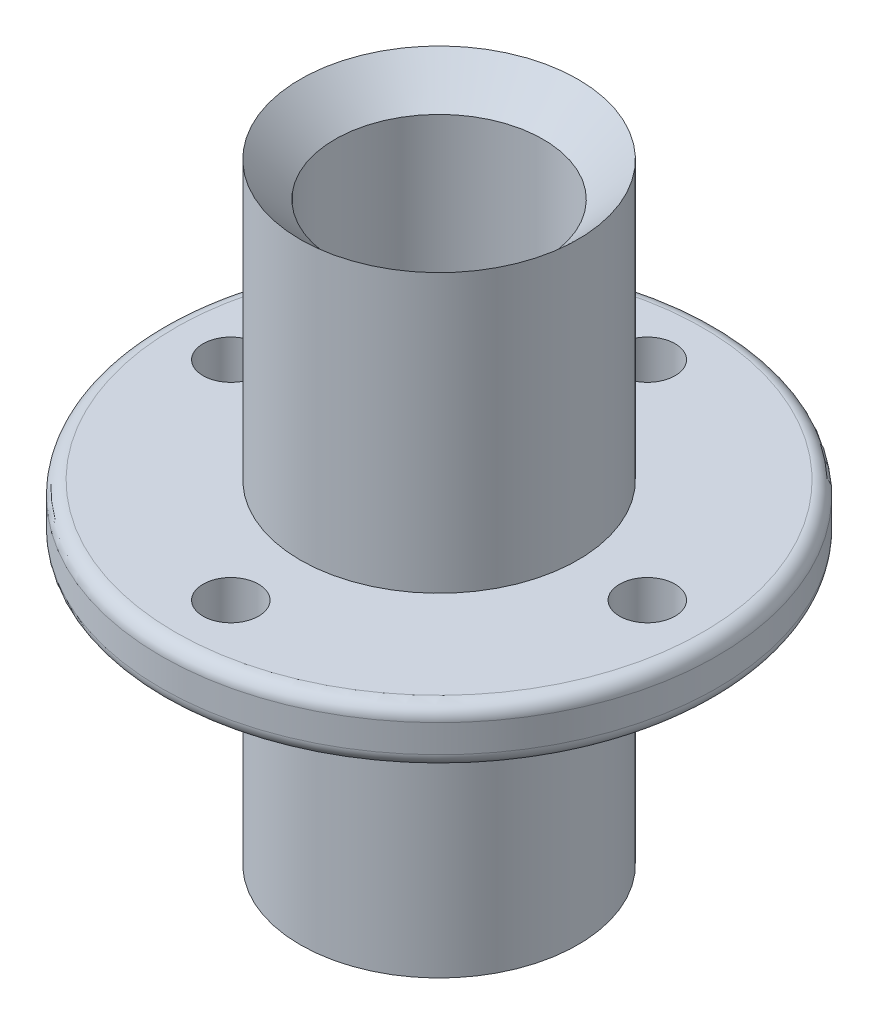
ISO-10303-21;
HEADER;
FILE_DESCRIPTION(('STEP AP214'),'2;1');
FILE_NAME('part.step','',(''),(''),'','','');
FILE_SCHEMA(('AUTOMOTIVE_DESIGN { 1 0 10303 214 1 1 1 1 }'));
ENDSEC;
DATA;
#1=APPLICATION_CONTEXT('core data for automotive mechanical design processes');
#2=APPLICATION_PROTOCOL_DEFINITION('international standard','automotive_design',2000,#1);
#3=PRODUCT_CONTEXT('',#1,'mechanical');
#4=PRODUCT('Part','Part','',(#3));
#5=PRODUCT_RELATED_PRODUCT_CATEGORY('part','',(#4));
#6=PRODUCT_DEFINITION_FORMATION('','',#4);
#7=PRODUCT_DEFINITION_CONTEXT('part definition',#1,'design');
#8=PRODUCT_DEFINITION('design','',#6,#7);
#9=PRODUCT_DEFINITION_SHAPE('','',#8);
#10=(LENGTH_UNIT() NAMED_UNIT(*) SI_UNIT(.MILLI.,.METRE.));
#11=(NAMED_UNIT(*) PLANE_ANGLE_UNIT() SI_UNIT($,.RADIAN.));
#12=(NAMED_UNIT(*) SI_UNIT($,.STERADIAN.) SOLID_ANGLE_UNIT());
#13=UNCERTAINTY_MEASURE_WITH_UNIT(LENGTH_MEASURE(1.E-05),#10,'distance_accuracy_value','');
#14=(GEOMETRIC_REPRESENTATION_CONTEXT(3) GLOBAL_UNCERTAINTY_ASSIGNED_CONTEXT((#13)) GLOBAL_UNIT_ASSIGNED_CONTEXT((#10,
#11,#12)) REPRESENTATION_CONTEXT('',''));
#15=CARTESIAN_POINT('',(0.,0.,0.));
#16=DIRECTION('',(0.,0.,1.));
#17=DIRECTION('',(1.,0.,0.));
#18=AXIS2_PLACEMENT_3D('',#15,#16,#17);
#19=CARTESIAN_POINT('',(0.,88.,0.));
#20=DIRECTION('',(0.,-1.,0.));
#21=DIRECTION('',(0.,0.,-1.));
#22=AXIS2_PLACEMENT_3D('',#19,#20,#21);
#23=CYLINDRICAL_SURFACE('',#22,20.);
#24=CARTESIAN_POINT('',(0.,0.,0.));
#25=DIRECTION('',(0.,1.,0.));
#26=DIRECTION('',(0.,0.,1.));
#27=AXIS2_PLACEMENT_3D('',#24,#25,#26);
#28=CIRCLE('',#27,20.);
#29=CARTESIAN_POINT('',(0.,0.,20.));
#30=VERTEX_POINT('',#29);
#31=EDGE_CURVE('E84',#30,#30,#28,.T.);
#32=ORIENTED_EDGE('',*,*,#31,.T.);
#33=EDGE_LOOP('',(#32));
#34=FACE_BOUND('',#33,.T.);
#35=CARTESIAN_POINT('',(0.,40.,0.));
#36=DIRECTION('',(0.,1.,0.));
#37=DIRECTION('',(0.,0.,1.));
#38=AXIS2_PLACEMENT_3D('',#35,#36,#37);
#39=CIRCLE('',#38,20.);
#40=CARTESIAN_POINT('',(0.,40.,20.));
#41=VERTEX_POINT('',#40);
#42=EDGE_CURVE('E81',#41,#41,#39,.T.);
#43=ORIENTED_EDGE('',*,*,#42,.F.);
#44=EDGE_LOOP('',(#43));
#45=FACE_BOUND('',#44,.T.);
#46=ADVANCED_FACE('F44',(#34,#45),#23,.T.);
#47=CARTESIAN_POINT('',(0.,0.,0.));
#48=DIRECTION('',(0.,1.,0.));
#49=DIRECTION('',(0.,0.,1.));
#50=AXIS2_PLACEMENT_3D('',#47,#48,#49);
#51=PLANE('',#50);
#52=ORIENTED_EDGE('',*,*,#31,.F.);
#53=EDGE_LOOP('',(#52));
#54=FACE_BOUND('',#53,.T.);
#55=ADVANCED_FACE('F114',(#54),#51,.F.);
#56=CARTESIAN_POINT('',(0.,48.,0.));
#57=DIRECTION('',(0.,1.,0.));
#58=DIRECTION('',(0.,0.,1.));
#59=AXIS2_PLACEMENT_3D('',#56,#57,#58);
#60=PLANE('',#59);
#61=CARTESIAN_POINT('',(0.,48.,-30.));
#62=DIRECTION('',(0.,1.,0.));
#63=DIRECTION('',(0.,0.,1.));
#64=AXIS2_PLACEMENT_3D('',#61,#62,#63);
#65=CIRCLE('',#64,4.);
#66=CARTESIAN_POINT('',(0.,48.,-26.));
#67=VERTEX_POINT('',#66);
#68=EDGE_CURVE('E68',#67,#67,#65,.T.);
#69=ORIENTED_EDGE('',*,*,#68,.F.);
#70=EDGE_LOOP('',(#69));
#71=FACE_BOUND('',#70,.T.);
#72=CARTESIAN_POINT('',(30.,48.,0.));
#73=DIRECTION('',(0.,1.,0.));
#74=DIRECTION('',(0.,0.,1.));
#75=AXIS2_PLACEMENT_3D('',#72,#73,#74);
#76=CIRCLE('',#75,4.00000000000001);
#77=CARTESIAN_POINT('',(30.,48.,4.00000000000001));
#78=VERTEX_POINT('',#77);
#79=EDGE_CURVE('E192',#78,#78,#76,.T.);
#80=ORIENTED_EDGE('',*,*,#79,.F.);
#81=EDGE_LOOP('',(#80));
#82=FACE_BOUND('',#81,.T.);
#83=CARTESIAN_POINT('',(0.,48.,30.));
#84=DIRECTION('',(0.,1.,0.));
#85=DIRECTION('',(0.,0.,1.));
#86=AXIS2_PLACEMENT_3D('',#83,#84,#85);
#87=CIRCLE('',#86,4.);
#88=CARTESIAN_POINT('',(0.,48.,34.));
#89=VERTEX_POINT('',#88);
#90=EDGE_CURVE('E193',#89,#89,#87,.T.);
#91=ORIENTED_EDGE('',*,*,#90,.F.);
#92=EDGE_LOOP('',(#91));
#93=FACE_BOUND('',#92,.T.);
#94=CARTESIAN_POINT('',(-30.,48.,0.));
#95=DIRECTION('',(0.,1.,0.));
#96=DIRECTION('',(0.,0.,1.));
#97=AXIS2_PLACEMENT_3D('',#94,#95,#96);
#98=CIRCLE('',#97,4.);
#99=CARTESIAN_POINT('',(-30.,48.,4.));
#100=VERTEX_POINT('',#99);
#101=EDGE_CURVE('E184',#100,#100,#98,.T.);
#102=ORIENTED_EDGE('',*,*,#101,.F.);
#103=EDGE_LOOP('',(#102));
#104=FACE_BOUND('',#103,.T.);
#105=CARTESIAN_POINT('',(0.,48.,0.));
#106=DIRECTION('',(0.,1.,0.));
#107=DIRECTION('',(0.,0.,1.));
#108=AXIS2_PLACEMENT_3D('',#105,#106,#107);
#109=CIRCLE('',#108,38.);
#110=CARTESIAN_POINT('',(0.,48.,38.));
#111=VERTEX_POINT('',#110);
#112=EDGE_CURVE('E96',#111,#111,#109,.T.);
#113=ORIENTED_EDGE('',*,*,#112,.T.);
#114=EDGE_LOOP('',(#113));
#115=FACE_BOUND('',#114,.T.);
#116=CARTESIAN_POINT('',(0.,48.,0.));
#117=DIRECTION('',(0.,1.,0.));
#118=DIRECTION('',(0.,0.,1.));
#119=AXIS2_PLACEMENT_3D('',#116,#117,#118);
#120=CIRCLE('',#119,20.);
#121=CARTESIAN_POINT('',(0.,48.,20.));
#122=VERTEX_POINT('',#121);
#123=EDGE_CURVE('E71',#122,#122,#120,.T.);
#124=ORIENTED_EDGE('',*,*,#123,.F.);
#125=EDGE_LOOP('',(#124));
#126=FACE_BOUND('',#125,.T.);
#127=ADVANCED_FACE('F108',(#71,#82,#93,#104,#115,#126),#60,.T.);
#128=CARTESIAN_POINT('',(0.,40.,0.));
#129=DIRECTION('',(0.,1.,0.));
#130=DIRECTION('',(0.,0.,1.));
#131=AXIS2_PLACEMENT_3D('',#128,#129,#130);
#132=PLANE('',#131);
#133=CARTESIAN_POINT('',(0.,40.,-30.));
#134=DIRECTION('',(0.,1.,0.));
#135=DIRECTION('',(0.,0.,1.));
#136=AXIS2_PLACEMENT_3D('',#133,#134,#135);
#137=CIRCLE('',#136,4.);
#138=CARTESIAN_POINT('',(0.,40.,-26.));
#139=VERTEX_POINT('',#138);
#140=EDGE_CURVE('E47',#139,#139,#137,.T.);
#141=ORIENTED_EDGE('',*,*,#140,.T.);
#142=EDGE_LOOP('',(#141));
#143=FACE_BOUND('',#142,.T.);
#144=CARTESIAN_POINT('',(30.,40.,0.));
#145=DIRECTION('',(0.,1.,0.));
#146=DIRECTION('',(0.,0.,1.));
#147=AXIS2_PLACEMENT_3D('',#144,#145,#146);
#148=CIRCLE('',#147,4.00000000000001);
#149=CARTESIAN_POINT('',(30.,40.,4.00000000000001));
#150=VERTEX_POINT('',#149);
#151=EDGE_CURVE('E67',#150,#150,#148,.T.);
#152=ORIENTED_EDGE('',*,*,#151,.T.);
#153=EDGE_LOOP('',(#152));
#154=FACE_BOUND('',#153,.T.);
#155=CARTESIAN_POINT('',(0.,40.,30.));
#156=DIRECTION('',(0.,1.,0.));
#157=DIRECTION('',(0.,0.,1.));
#158=AXIS2_PLACEMENT_3D('',#155,#156,#157);
#159=CIRCLE('',#158,4.);
#160=CARTESIAN_POINT('',(0.,40.,34.));
#161=VERTEX_POINT('',#160);
#162=EDGE_CURVE('E62',#161,#161,#159,.T.);
#163=ORIENTED_EDGE('',*,*,#162,.T.);
#164=EDGE_LOOP('',(#163));
#165=FACE_BOUND('',#164,.T.);
#166=CARTESIAN_POINT('',(-30.,40.,0.));
#167=DIRECTION('',(0.,1.,0.));
#168=DIRECTION('',(0.,0.,1.));
#169=AXIS2_PLACEMENT_3D('',#166,#167,#168);
#170=CIRCLE('',#169,4.);
#171=CARTESIAN_POINT('',(-30.,40.,4.));
#172=VERTEX_POINT('',#171);
#173=EDGE_CURVE('E65',#172,#172,#170,.T.);
#174=ORIENTED_EDGE('',*,*,#173,.T.);
#175=EDGE_LOOP('',(#174));
#176=FACE_BOUND('',#175,.T.);
#177=CARTESIAN_POINT('',(0.,40.,0.));
#178=DIRECTION('',(0.,1.,0.));
#179=DIRECTION('',(0.,0.,1.));
#180=AXIS2_PLACEMENT_3D('',#177,#178,#179);
#181=CIRCLE('',#180,38.);
#182=CARTESIAN_POINT('',(0.,40.,38.));
#183=VERTEX_POINT('',#182);
#184=EDGE_CURVE('E10',#183,#183,#181,.F.);
#185=ORIENTED_EDGE('',*,*,#184,.T.);
#186=EDGE_LOOP('',(#185));
#187=FACE_BOUND('',#186,.T.);
#188=ORIENTED_EDGE('',*,*,#42,.T.);
#189=EDGE_LOOP('',(#188));
#190=FACE_BOUND('',#189,.T.);
#191=ADVANCED_FACE('F115',(#143,#154,#165,#176,#187,#190),#132,.F.);
#192=CARTESIAN_POINT('',(0.,48.,0.));
#193=DIRECTION('',(0.,-1.,0.));
#194=DIRECTION('',(0.,0.,-1.));
#195=AXIS2_PLACEMENT_3D('',#192,#193,#194);
#196=CYLINDRICAL_SURFACE('',#195,40.);
#197=CARTESIAN_POINT('',(0.,42.,0.));
#198=DIRECTION('',(0.,1.,0.));
#199=DIRECTION('',(0.,0.,1.));
#200=AXIS2_PLACEMENT_3D('',#197,#198,#199);
#201=CIRCLE('',#200,40.);
#202=CARTESIAN_POINT('',(0.,42.,40.));
#203=VERTEX_POINT('',#202);
#204=EDGE_CURVE('E52',#203,#203,#201,.T.);
#205=ORIENTED_EDGE('',*,*,#204,.T.);
#206=EDGE_LOOP('',(#205));
#207=FACE_BOUND('',#206,.T.);
#208=CARTESIAN_POINT('',(0.,46.,0.));
#209=DIRECTION('',(0.,1.,0.));
#210=DIRECTION('',(0.,0.,1.));
#211=AXIS2_PLACEMENT_3D('',#208,#209,#210);
#212=CIRCLE('',#211,40.);
#213=CARTESIAN_POINT('',(0.,46.,40.));
#214=VERTEX_POINT('',#213);
#215=EDGE_CURVE('E59',#214,#214,#212,.F.);
#216=ORIENTED_EDGE('',*,*,#215,.T.);
#217=EDGE_LOOP('',(#216));
#218=FACE_BOUND('',#217,.T.);
#219=ADVANCED_FACE('F101',(#207,#218),#196,.T.);
#220=ORIENTED_EDGE('',*,*,#123,.T.);
#221=EDGE_LOOP('',(#220));
#222=FACE_BOUND('',#221,.T.);
#223=CARTESIAN_POINT('',(0.,88.,0.));
#224=DIRECTION('',(0.,1.,0.));
#225=DIRECTION('',(0.,0.,1.));
#226=AXIS2_PLACEMENT_3D('',#223,#224,#225);
#227=CIRCLE('',#226,20.);
#228=CARTESIAN_POINT('',(0.,88.,20.));
#229=VERTEX_POINT('',#228);
#230=EDGE_CURVE('E86',#229,#229,#227,.T.);
#231=ORIENTED_EDGE('',*,*,#230,.F.);
#232=EDGE_LOOP('',(#231));
#233=FACE_BOUND('',#232,.T.);
#234=ADVANCED_FACE('F128',(#222,#233),#23,.T.);
#235=CARTESIAN_POINT('',(0.,83.,0.));
#236=DIRECTION('',(0.,1.,0.));
#237=DIRECTION('',(0.,0.,1.));
#238=AXIS2_PLACEMENT_3D('',#235,#236,#237);
#239=CONICAL_SURFACE('',#238,15.,0.78539816339745);
#240=ORIENTED_EDGE('',*,*,#230,.T.);
#241=EDGE_LOOP('',(#240));
#242=FACE_BOUND('',#241,.T.);
#243=CARTESIAN_POINT('',(0.,83.,0.));
#244=DIRECTION('',(0.,1.,0.));
#245=DIRECTION('',(0.,0.,1.));
#246=AXIS2_PLACEMENT_3D('',#243,#244,#245);
#247=CIRCLE('',#246,15.);
#248=CARTESIAN_POINT('',(0.,83.,15.));
#249=VERTEX_POINT('',#248);
#250=EDGE_CURVE('E93',#249,#249,#247,.T.);
#251=ORIENTED_EDGE('',*,*,#250,.F.);
#252=EDGE_LOOP('',(#251));
#253=FACE_BOUND('',#252,.T.);
#254=ADVANCED_FACE('F139',(#242,#253),#239,.F.);
#255=CARTESIAN_POINT('',(0.,4.99999999999999,0.));
#256=DIRECTION('',(0.,1.,0.));
#257=DIRECTION('',(0.,0.,1.));
#258=AXIS2_PLACEMENT_3D('',#255,#256,#257);
#259=CYLINDRICAL_SURFACE('',#258,15.);
#260=ORIENTED_EDGE('',*,*,#250,.T.);
#261=EDGE_LOOP('',(#260));
#262=FACE_BOUND('',#261,.T.);
#263=CARTESIAN_POINT('',(0.,4.99999999999999,0.));
#264=DIRECTION('',(0.,1.,0.));
#265=DIRECTION('',(0.,0.,1.));
#266=AXIS2_PLACEMENT_3D('',#263,#264,#265);
#267=CIRCLE('',#266,15.);
#268=CARTESIAN_POINT('',(0.,4.99999999999999,15.));
#269=VERTEX_POINT('',#268);
#270=EDGE_CURVE('E80',#269,#269,#267,.T.);
#271=ORIENTED_EDGE('',*,*,#270,.F.);
#272=EDGE_LOOP('',(#271));
#273=FACE_BOUND('',#272,.T.);
#274=ADVANCED_FACE('F106',(#262,#273),#259,.F.);
#275=CARTESIAN_POINT('',(0.,46.,0.));
#276=DIRECTION('',(0.,1.,0.));
#277=DIRECTION('',(0.,0.,1.));
#278=AXIS2_PLACEMENT_3D('',#275,#276,#277);
#279=TOROIDAL_SURFACE('',#278,38.,2.);
#280=ORIENTED_EDGE('',*,*,#215,.F.);
#281=EDGE_LOOP('',(#280));
#282=FACE_BOUND('',#281,.T.);
#283=ORIENTED_EDGE('',*,*,#112,.F.);
#284=EDGE_LOOP('',(#283));
#285=FACE_BOUND('',#284,.T.);
#286=ADVANCED_FACE('F103',(#282,#285),#279,.T.);
#287=CARTESIAN_POINT('',(0.,42.,0.));
#288=DIRECTION('',(0.,1.,0.));
#289=DIRECTION('',(0.,0.,1.));
#290=AXIS2_PLACEMENT_3D('',#287,#288,#289);
#291=TOROIDAL_SURFACE('',#290,38.,2.);
#292=ORIENTED_EDGE('',*,*,#184,.F.);
#293=EDGE_LOOP('',(#292));
#294=FACE_BOUND('',#293,.T.);
#295=ORIENTED_EDGE('',*,*,#204,.F.);
#296=EDGE_LOOP('',(#295));
#297=FACE_BOUND('',#296,.T.);
#298=ADVANCED_FACE('F50',(#294,#297),#291,.T.);
#299=CARTESIAN_POINT('',(-30.,29.,0.));
#300=DIRECTION('',(0.,1.,0.));
#301=DIRECTION('',(0.,0.,1.));
#302=AXIS2_PLACEMENT_3D('',#299,#300,#301);
#303=CYLINDRICAL_SURFACE('',#302,4.);
#304=ORIENTED_EDGE('',*,*,#101,.T.);
#305=EDGE_LOOP('',(#304));
#306=FACE_BOUND('',#305,.T.);
#307=ORIENTED_EDGE('',*,*,#173,.F.);
#308=EDGE_LOOP('',(#307));
#309=FACE_BOUND('',#308,.T.);
#310=ADVANCED_FACE('F174',(#306,#309),#303,.F.);
#311=CARTESIAN_POINT('',(0.,29.,30.));
#312=DIRECTION('',(0.,1.,0.));
#313=DIRECTION('',(0.,0.,1.));
#314=AXIS2_PLACEMENT_3D('',#311,#312,#313);
#315=CYLINDRICAL_SURFACE('',#314,4.);
#316=ORIENTED_EDGE('',*,*,#90,.T.);
#317=EDGE_LOOP('',(#316));
#318=FACE_BOUND('',#317,.T.);
#319=ORIENTED_EDGE('',*,*,#162,.F.);
#320=EDGE_LOOP('',(#319));
#321=FACE_BOUND('',#320,.T.);
#322=ADVANCED_FACE('F170',(#318,#321),#315,.F.);
#323=CARTESIAN_POINT('',(30.,29.,0.));
#324=DIRECTION('',(0.,1.,0.));
#325=DIRECTION('',(0.,0.,1.));
#326=AXIS2_PLACEMENT_3D('',#323,#324,#325);
#327=CYLINDRICAL_SURFACE('',#326,4.00000000000001);
#328=ORIENTED_EDGE('',*,*,#79,.T.);
#329=EDGE_LOOP('',(#328));
#330=FACE_BOUND('',#329,.T.);
#331=ORIENTED_EDGE('',*,*,#151,.F.);
#332=EDGE_LOOP('',(#331));
#333=FACE_BOUND('',#332,.T.);
#334=ADVANCED_FACE('F161',(#330,#333),#327,.F.);
#335=CARTESIAN_POINT('',(0.,29.,-30.));
#336=DIRECTION('',(0.,1.,0.));
#337=DIRECTION('',(0.,0.,1.));
#338=AXIS2_PLACEMENT_3D('',#335,#336,#337);
#339=CYLINDRICAL_SURFACE('',#338,4.);
#340=ORIENTED_EDGE('',*,*,#68,.T.);
#341=EDGE_LOOP('',(#340));
#342=FACE_BOUND('',#341,.T.);
#343=ORIENTED_EDGE('',*,*,#140,.F.);
#344=EDGE_LOOP('',(#343));
#345=FACE_BOUND('',#344,.T.);
#346=ADVANCED_FACE('F156',(#342,#345),#339,.F.);
#347=CARTESIAN_POINT('',(0.,4.99999999999999,0.));
#348=DIRECTION('',(0.,1.,0.));
#349=DIRECTION('',(0.,0.,1.));
#350=AXIS2_PLACEMENT_3D('',#347,#348,#349);
#351=PLANE('',#350);
#352=ORIENTED_EDGE('',*,*,#270,.T.);
#353=EDGE_LOOP('',(#352));
#354=FACE_BOUND('',#353,.T.);
#355=ADVANCED_FACE('F152',(#354),#351,.T.);
#356=CLOSED_SHELL('',(#46,#55,#127,#191,#219,#234,#254,#274,#286,#298,#310,#322,#334,#346,#355));
#357=MANIFOLD_SOLID_BREP('B2',#356);
#358=ADVANCED_BREP_SHAPE_REPRESENTATION('',(#18,#357),#14);
#359=SHAPE_DEFINITION_REPRESENTATION(#9,#358);
ENDSEC;
END-ISO-10303-21;
